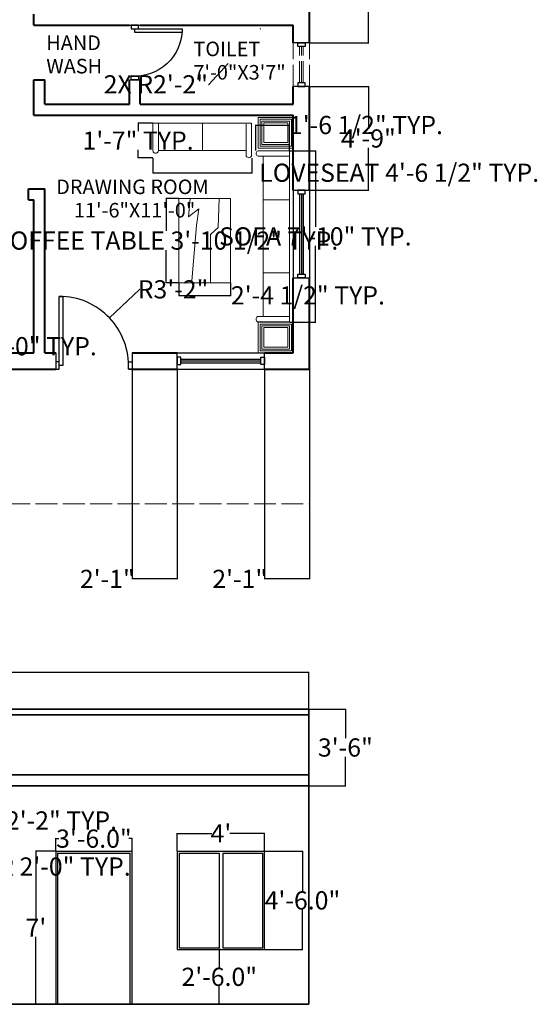
# Model space of a CAD drawing. Units: inches. Extents: x -413 to 212, y 1694 to 2633.
# Tile 3 of 5: x -98 to 187, y 1738 to 2279. Entities that reach past the tile are written whole.
import ezdxf

# ---------------------------------------------------------------- set-up
doc = ezdxf.new("R2010")
doc.units = ezdxf.units.IN
doc.header["$MEASUREMENT"] = 0
doc.linetypes.add('ACAD_ISO02W100', pattern=[15, 12, -3])
for name, color, linetype, lineweight in [('A-ANNO-DIMS', 5, 'Continuous', 18), ('A-AREA-IDEN', 251, 'Continuous', 25), ('A-ELEV', 20, 'Continuous', 35), ('A-ELEV-DOOR', 4, 'Continuous', 25), ('A-ELEV-GLAZ', 6, 'Continuous', 25), ('A-FLOR-OVHD', 20, 'ACAD_ISO02W100', 18), ('A-GLAZ-OVHD', 2, 'ACAD_ISO02W100', 18), ('A-GLAZ-VENT', 2, 'Continuous', 25), ('door', 4, 'Continuous', 25), ('furniture', 1, 'Continuous', 18), ('wall', 20, 'Continuous', 40), ('window', 6, 'Continuous', 25)]:
    doc.layers.add(name, color=color, linetype=linetype, lineweight=lineweight)
doc.styles.get("Standard").update_dxf_attribs({"font": 'arial.ttf'})
doc.dimstyles.get("Standard").update_dxf_attribs({"dimtxt": 10, "dimasz": 0.18, "dimexe": 0.18, "dimexo": 0.0625, "dimgap": 0.09, "dimtad": 0, "dimtih": 1, "dimtoh": 1, "dimdec": 1, "dimzin": 0, "dimdsep": 46, "dimlunit": 3, "dimtxsty": 'Standard', "dimblk": 'ARCHTICK', "dimcen": 0.09, "dimadec": 0, "dimazin": 0, "dimtfac": 1, "dimtdec": 1, "dimtofl": 0, "dimtmove": 0, "dimatfit": 3, "dimfxl": 1, "dimtolj": 1, "dimtzin": 0, "dimarcsym": 0})

# ---------------------------------------------------------------- blocks, each defined once
blk = doc.blocks.new('_ArchTick')
at = {"color": 0, "linetype": 'ByBlock', "const_width": 0.15}
blk.add_lwpolyline([(-0.5, -0.5), (0.5, 0.5)], dxfattribs=at)
blk = doc.blocks.new('*D4')
at = {"layer": 'A-ANNO-DIMS', "color": 0, "lineweight": -2, "transparency": 16777216}
for p, q in [((12.71, 1768.59), (11.69, 1768.59)), ((11.87, 1768.59), (11.87, 1758.78)), ((11.87, 1738.59), (11.87, 1748.39)), ((12.71, 1738.59), (11.69, 1738.59))]:
    blk.add_line(p, q, dxfattribs=at)
at = {"layer": 'Defpoints', "color": 0, "transparency": 16777216}
for p in [(12.77, 1768.59), (11.87, 1738.59), (12.77, 1738.59)]:
    blk.add_point(p, dxfattribs=at)
at = {"layer": 'A-ANNO-DIMS', "color": 0, "lineweight": -2, "transparency": 16777216, "xscale": 0.18, "yscale": 0.18, "zscale": 0.18}
for p, rotation in [((11.87, 1768.59), 90), ((11.87, 1738.59), 270)]:
    blk.add_blockref('_ArchTick', p, dxfattribs=dict(at, rotation=rotation))
at = {"layer": 'A-ANNO-DIMS', "color": 0, "transparency": 16777216, "insert": (11.87, 1753.59), "char_height": 10, "attachment_point": 5}
blk.add_mtext('\\A1;2\'-6.0"', dxfattribs=at)
blk = doc.blocks.new('*D5')
at = {"layer": 'A-ANNO-DIMS', "color": 0, "lineweight": -2, "transparency": 16777216}
for p, q in [((-78.04, 1822.59), (-89.03, 1822.59)), ((-88.85, 1822.59), (-88.85, 1785.68)), ((-88.85, 1738.59), (-88.85, 1775.5)), ((-78.04, 1738.59), (-89.03, 1738.59))]:
    blk.add_line(p, q, dxfattribs=at)
at = {"layer": 'Defpoints', "color": 0, "transparency": 16777216}
for p in [(-77.98, 1822.59), (-88.85, 1738.59), (-77.98, 1738.59)]:
    blk.add_point(p, dxfattribs=at)
at = {"layer": 'A-ANNO-DIMS', "color": 0, "lineweight": -2, "transparency": 16777216, "xscale": 0.18, "yscale": 0.18, "zscale": 0.18}
for p, rotation in [((-88.85, 1822.59), 90), ((-88.85, 1738.59), 270)]:
    blk.add_blockref('_ArchTick', p, dxfattribs=dict(at, rotation=rotation))
at = {"layer": 'A-ANNO-DIMS', "color": 0, "transparency": 16777216, "insert": (-88.85, 1780.59), "char_height": 10, "attachment_point": 5}
blk.add_mtext("\\A1;7'", dxfattribs=at)
blk = doc.blocks.new('*D6')
at = {"layer": 'A-ANNO-DIMS', "color": 0, "lineweight": -2, "transparency": 16777216}
for p, q in [((-77.98, 1822.65), (-77.98, 1829.7)), ((-77.98, 1829.52), (-76.18, 1829.52)), ((-35.98, 1829.52), (-37.77, 1829.52)), ((-35.98, 1822.65), (-35.98, 1829.7))]:
    blk.add_line(p, q, dxfattribs=at)
at = {"layer": 'Defpoints', "color": 0, "transparency": 16777216}
for p in [(-77.98, 1829.52), (-77.98, 1822.59), (-35.98, 1822.59)]:
    blk.add_point(p, dxfattribs=at)
at = {"layer": 'A-ANNO-DIMS', "color": 0, "lineweight": -2, "transparency": 16777216, "xscale": 0.18, "yscale": 0.18, "zscale": 0.18, "rotation": 180}
blk.add_blockref('_ArchTick', (-77.98, 1829.52), dxfattribs=at)
at = {"layer": 'A-ANNO-DIMS', "color": 0, "lineweight": -2, "transparency": 16777216, "xscale": 0.18, "yscale": 0.18, "zscale": 0.18}
blk.add_blockref('_ArchTick', (-35.98, 1829.52), dxfattribs=at)
at = {"layer": 'A-ANNO-DIMS', "color": 0, "transparency": 16777216, "insert": (-56.98, 1829.52), "char_height": 10, "attachment_point": 5}
blk.add_mtext('\\A1;3\'-6.0"', dxfattribs=at)
blk = doc.blocks.new('*D7')
at = {"layer": 'A-ANNO-DIMS', "color": 0, "lineweight": -2, "transparency": 16777216}
for p, q in [((36.84, 1822.59), (57.74, 1822.59)), ((57.56, 1822.59), (57.56, 1800.78)), ((57.56, 1768.59), (57.56, 1790.39)), ((36.84, 1768.59), (57.74, 1768.59))]:
    blk.add_line(p, q, dxfattribs=at)
at = {"layer": 'Defpoints', "color": 0, "transparency": 16777216}
for p in [(36.77, 1822.59), (36.77, 1768.59), (57.56, 1768.59)]:
    blk.add_point(p, dxfattribs=at)
at = {"layer": 'A-ANNO-DIMS', "color": 0, "lineweight": -2, "transparency": 16777216, "xscale": 0.18, "yscale": 0.18, "zscale": 0.18}
for p, rotation in [((57.56, 1822.59), 90), ((57.56, 1768.59), 270)]:
    blk.add_blockref('_ArchTick', p, dxfattribs=dict(at, rotation=rotation))
at = {"layer": 'A-ANNO-DIMS', "color": 0, "transparency": 16777216, "insert": (57.56, 1795.59), "char_height": 10, "attachment_point": 5}
blk.add_mtext('\\A1;4\'-6.0"', dxfattribs=at)
blk = doc.blocks.new('*D8')
at = {"layer": 'A-ANNO-DIMS', "color": 0, "lineweight": -2, "transparency": 16777216}
for p, q in [((-11.23, 1822.65), (-11.23, 1832.6)), ((-11.23, 1832.42), (7.88, 1832.42)), ((36.77, 1832.42), (17.67, 1832.42)), ((36.77, 1822.65), (36.77, 1832.6))]:
    blk.add_line(p, q, dxfattribs=at)
at = {"layer": 'Defpoints', "color": 0, "transparency": 16777216}
for p in [(-11.23, 1832.42), (-11.23, 1822.59), (36.77, 1822.59)]:
    blk.add_point(p, dxfattribs=at)
at = {"layer": 'A-ANNO-DIMS', "color": 0, "lineweight": -2, "transparency": 16777216, "xscale": 0.18, "yscale": 0.18, "zscale": 0.18, "rotation": 180}
blk.add_blockref('_ArchTick', (-11.23, 1832.42), dxfattribs=at)
at = {"layer": 'A-ANNO-DIMS', "color": 0, "lineweight": -2, "transparency": 16777216, "xscale": 0.18, "yscale": 0.18, "zscale": 0.18}
blk.add_blockref('_ArchTick', (36.77, 1832.42), dxfattribs=at)
at = {"layer": 'A-ANNO-DIMS', "color": 0, "transparency": 16777216, "insert": (12.77, 1832.42), "char_height": 10, "attachment_point": 5}
blk.add_mtext("\\A1;4'", dxfattribs=at)
blk = doc.blocks.new('WINDOW-48IN')
for p, q in [((0, 0), (0, 9)), ((0, 9), (48, 9)), ((2, 5.5), (46, 5.5)), ((48, 0), (48, 9)), ((2, 4.5), (46, 4.5)), ((2, 3.5), (46, 3.5)), ((0, 0), (48, 0))]:
    blk.add_line(p, q)
for points in [[(0, 2.5), (2, 2.5), (2, 6.5), (0, 6.5)], [(48, 2.5), (46, 2.5), (46, 6.5), (48, 6.5)]]:
    blk.add_lwpolyline(points, close=True)
blk = doc.blocks.new('VENT-JAMBS-24IN')
for p, q in [((0, 0), (0, 9)), ((24, 0), (24, 9))]:
    blk.add_line(p, q)
for points in [[(0, 2.5), (2, 2.5), (2, 6.5), (0, 6.5)], [(24, 2.5), (22, 2.5), (22, 6.5), (24, 6.5)]]:
    blk.add_lwpolyline(points, close=True)
blk = doc.blocks.new('VENT-PANEL-24IN')
for p, q in [((0, 9), (24, 9)), ((2, 5.5), (22, 5.5)), ((2, 4.5), (22, 4.5)), ((2, 3.5), (22, 3.5)), ((0, 0), (24, 0))]:
    blk.add_line(p, q)
blk = doc.blocks.new('DOOR-SWING-30IN')
for points in [[(0, 0), (0, 26), (-2, 26), (-2, 0)], [(-28, -2), (-26, -2), (-26, 2), (-28, 2)], [(2, -2), (0, -2), (0, 2), (2, 2)]]:
    blk.add_lwpolyline(points, close=True)
blk.add_arc((0, 0), 26, 90, 184.4117)
blk = doc.blocks.new('SOFA-THREE-SEAT')
for points in [[(0, 1.47), (0, 18.46), (94.05, 18.46), (94.05, 1.28)], [(3, 1.47), (3, 18.46)], [(27, 4), (27, 18.46)], [(67.05, 18.46), (67.05, 4)], [(91.05, 18.46), (91.05, 1.28)], [(91.05, 4), (3, 4)]]:
    blk.add_lwpolyline(points)
for centre, radius, start, end in [((1.5, 1.51), 1.5, 178.5982, 1.4018), ((92.55, 1.52), 1.52, 171.0874, 8.9126)]:
    blk.add_arc(centre, radius, start, end)
blk = doc.blocks.new('SOFA-TWO-SEAT')
for points in [[(0, 0), (0, 54.18), (17.18, 54.18)], [(0.47, 51.18), (17.65, 51.18)], [(14.93, 51.18), (14.93, 3.18)], [(0, 27.18), (14.93, 27.18)], [(15.01, 3), (0, 3)], [(0, 0), (14.93, 0)]]:
    blk.add_lwpolyline(points)
for centre, radius, start, end in [((17.41, 52.68), 1.52, 261.0874, 98.9126), ((14.97, 1.5), 1.5, 268.5982, 91.4018)]:
    blk.add_arc(centre, radius, start, end)
blk = doc.blocks.new('TABLE-COFFEE')
for p, q in [((0, 22.18), (0, 22.18)), ((0, 22.18), (15.93, 21.7)), ((15.93, 21.7), (19.8, 17.36)), ((19.8, 17.36), (46.35, 17.36)), ((10.14, 5.3), (5.79, 11.09)), ((5.79, 11.09), (14.97, 9.64)), ((0, 6.27), (0, 6.27)), ((0, 6.27), (10.14, 5.3)), ((14.97, 9.64), (45.38, 7.23))]:
    blk.add_line(p, q)
blk.add_lwpolyline([(0, 28.45), (46.35, 28.45), (46.35, 0), (0, 0)], close=True)
blk = doc.blocks.new('TABLE-END')
for points in [[(0, 19.24), (16.8, 19.24), (16.8, 0), (0, 0)], [(1, 18.24), (15.8, 18.24), (15.8, 1), (1, 1)], [(2, 17.24), (14.8, 17.24), (14.8, 2), (2, 2)], [(3, 16.24), (13.8, 16.24), (13.8, 3), (3, 3)]]:
    blk.add_lwpolyline(points, close=True)
blk = doc.blocks.new('*D31')
at = {"layer": 'A-ANNO-DIMS', "color": 0, "lineweight": -2, "transparency": 16777216}
for p, q in [((-179.98, 2096.55), (-179.98, 2100.26)), ((-179.98, 2100.08), (-155.98, 2100.08)), ((-155.98, 2096.55), (-155.98, 2100.26)), ((-155.98, 2100.08), (-155.8, 2100.08))]:
    blk.add_line(p, q, dxfattribs=at)
at = {"layer": 'Defpoints', "color": 0, "transparency": 16777216}
for p in [(-155.98, 2100.08), (-179.98, 2096.48), (-155.98, 2096.48)]:
    blk.add_point(p, dxfattribs=at)
at = {"layer": 'A-ANNO-DIMS', "color": 0, "lineweight": -2, "transparency": 16777216, "xscale": 0.18, "yscale": 0.18, "zscale": 0.18, "rotation": 180}
blk.add_blockref('_ArchTick', (-179.98, 2100.08), dxfattribs=at)
at = {"layer": 'A-ANNO-DIMS', "color": 0, "lineweight": -2, "transparency": 16777216, "xscale": 0.18, "yscale": 0.18, "zscale": 0.18}
blk.add_blockref('_ArchTick', (-155.98, 2100.08), dxfattribs=at)
at = {"layer": 'A-ANNO-DIMS', "color": 0, "transparency": 16777216, "insert": (-104.4, 2100.08), "char_height": 10, "attachment_point": 5}
blk.add_mtext('\\A1;VENT 2\'-0" TYP.', dxfattribs=at)
blk = doc.blocks.new('*D45')
at = {"layer": 'A-ANNO-DIMS', "color": 0, "lineweight": -2, "transparency": 16777216}
for p, q in [((50.59, 2207.49), (64.83, 2207.49)), ((64.65, 2207.49), (64.65, 2165.68)), ((64.65, 2113.33), (64.65, 2155.15)), ((50.59, 2113.33), (64.83, 2113.33))]:
    blk.add_line(p, q, dxfattribs=at)
at = {"layer": 'Defpoints', "color": 0, "transparency": 16777216}
for p in [(50.52, 2207.49), (50.52, 2113.33), (64.65, 2113.33)]:
    blk.add_point(p, dxfattribs=at)
at = {"layer": 'A-ANNO-DIMS', "color": 0, "lineweight": -2, "transparency": 16777216, "xscale": 0.18, "yscale": 0.18, "zscale": 0.18}
for p, rotation in [((64.65, 2207.49), 90), ((64.65, 2113.33), 270)]:
    blk.add_blockref('_ArchTick', p, dxfattribs=dict(at, rotation=rotation))
at = {"layer": 'A-ANNO-DIMS', "color": 0, "transparency": 16777216, "insert": (64.65, 2160.41), "char_height": 10, "attachment_point": 5}
blk.add_mtext('\\A1;SOFA 7\'-10" TYP.', dxfattribs=at)
blk = doc.blocks.new('*D46')
at = {"layer": 'A-ANNO-DIMS', "color": 0, "lineweight": -2, "transparency": 16777216}
for p, q in [((31.98, 2207.55), (31.98, 2221.79)), ((31.98, 2221.61), (50.52, 2221.61)), ((50.52, 2207.55), (50.52, 2221.79)), ((50.52, 2221.61), (50.7, 2221.61))]:
    blk.add_line(p, q, dxfattribs=at)
at = {"layer": 'Defpoints', "color": 0, "transparency": 16777216}
for p in [(50.52, 2221.61), (31.98, 2207.49), (50.52, 2207.49)]:
    blk.add_point(p, dxfattribs=at)
at = {"layer": 'A-ANNO-DIMS', "color": 0, "lineweight": -2, "transparency": 16777216, "xscale": 0.18, "yscale": 0.18, "zscale": 0.18, "rotation": 180}
blk.add_blockref('_ArchTick', (31.98, 2221.61), dxfattribs=at)
at = {"layer": 'A-ANNO-DIMS', "color": 0, "lineweight": -2, "transparency": 16777216, "xscale": 0.18, "yscale": 0.18, "zscale": 0.18}
blk.add_blockref('_ArchTick', (50.52, 2221.61), dxfattribs=at)
at = {"layer": 'A-ANNO-DIMS', "color": 0, "transparency": 16777216, "insert": (92.45, 2221.61), "char_height": 10, "attachment_point": 5}
blk.add_mtext('\\A1;1\'-6 1/2" TYP.', dxfattribs=at)
blk = doc.blocks.new('*D47')
at = {"layer": 'A-ANNO-DIMS', "color": 0, "lineweight": -2, "transparency": 16777216}
for p, q in [((-24.57, 2203.48), (-24.57, 2195.22)), ((29.72, 2203.48), (29.72, 2195.22)), ((-24.57, 2195.4), (29.72, 2195.4)), ((29.72, 2195.4), (29.9, 2195.4))]:
    blk.add_line(p, q, dxfattribs=at)
at = {"layer": 'Defpoints', "color": 0, "transparency": 16777216}
for p in [(-24.57, 2203.54), (29.72, 2203.54), (29.72, 2195.4)]:
    blk.add_point(p, dxfattribs=at)
at = {"layer": 'A-ANNO-DIMS', "color": 0, "lineweight": -2, "transparency": 16777216, "xscale": 0.18, "yscale": 0.18, "zscale": 0.18, "rotation": 180}
blk.add_blockref('_ArchTick', (-24.57, 2195.4), dxfattribs=at)
at = {"layer": 'A-ANNO-DIMS', "color": 0, "lineweight": -2, "transparency": 16777216, "xscale": 0.18, "yscale": 0.18, "zscale": 0.18}
blk.add_blockref('_ArchTick', (29.72, 2195.4), dxfattribs=at)
at = {"layer": 'A-ANNO-DIMS', "color": 0, "transparency": 16777216, "insert": (110.71, 2195.4), "char_height": 10, "attachment_point": 5}
blk.add_mtext('\\A1;LOVESEAT 4\'-6 1/2" TYP.', dxfattribs=at)
blk = doc.blocks.new('*D48')
at = {"layer": 'A-ANNO-DIMS', "color": 0, "lineweight": -2, "transparency": 16777216}
for p, q in [((-24.63, 2222.56), (-32.89, 2222.56)), ((-32.71, 2222.56), (-32.71, 2218.16)), ((-32.71, 2203.54), (-32.71, 2207.94)), ((-24.63, 2203.54), (-32.89, 2203.54))]:
    blk.add_line(p, q, dxfattribs=at)
at = {"layer": 'Defpoints', "color": 0, "transparency": 16777216}
for p in [(-24.57, 2222.56), (-32.71, 2203.54), (-24.57, 2203.54)]:
    blk.add_point(p, dxfattribs=at)
at = {"layer": 'A-ANNO-DIMS', "color": 0, "lineweight": -2, "transparency": 16777216, "xscale": 0.18, "yscale": 0.18, "zscale": 0.18}
for p, rotation in [((-32.71, 2222.56), 90), ((-32.71, 2203.54), 270)]:
    blk.add_blockref('_ArchTick', p, dxfattribs=dict(at, rotation=rotation))
at = {"layer": 'A-ANNO-DIMS', "color": 0, "transparency": 16777216, "insert": (-32.71, 2213.05), "char_height": 10, "attachment_point": 5}
blk.add_mtext('\\A1;1\'-7" TYP.', dxfattribs=at)
blk = doc.blocks.new('*D49')
at = {"layer": 'A-ANNO-DIMS', "color": 0, "lineweight": -2, "transparency": 16777216}
for p, q in [((-10.42, 2181.31), (-17.49, 2181.31)), ((-17.31, 2181.31), (-17.31, 2163.4)), ((-17.31, 2134.96), (-17.31, 2152.87)), ((-10.42, 2134.96), (-17.49, 2134.96))]:
    blk.add_line(p, q, dxfattribs=at)
at = {"layer": 'Defpoints', "color": 0, "transparency": 16777216}
for p in [(-10.36, 2181.31), (-17.31, 2134.96), (-10.36, 2134.96)]:
    blk.add_point(p, dxfattribs=at)
at = {"layer": 'A-ANNO-DIMS', "color": 0, "lineweight": -2, "transparency": 16777216, "xscale": 0.18, "yscale": 0.18, "zscale": 0.18}
for p, rotation in [((-17.31, 2181.31), 90), ((-17.31, 2134.96), 270)]:
    blk.add_blockref('_ArchTick', p, dxfattribs=dict(at, rotation=rotation))
at = {"layer": 'A-ANNO-DIMS', "color": 0, "transparency": 16777216, "insert": (-17.31, 2158.13), "char_height": 10, "attachment_point": 5}
blk.add_mtext('\\A1;COFFEE TABLE 3\'-10 1/2" TYP.', dxfattribs=at)
blk = doc.blocks.new('*D50')
at = {"layer": 'A-ANNO-DIMS', "color": 0, "lineweight": -2, "transparency": 16777216}
for p, q in [((-10.36, 2134.9), (-10.36, 2127.83)), ((18.09, 2134.9), (18.09, 2127.83)), ((-10.36, 2128.01), (18.09, 2128.01)), ((18.09, 2128.01), (18.27, 2128.01))]:
    blk.add_line(p, q, dxfattribs=at)
at = {"layer": 'Defpoints', "color": 0, "transparency": 16777216}
for p in [(-10.36, 2134.96), (18.09, 2134.96), (18.09, 2128.01)]:
    blk.add_point(p, dxfattribs=at)
at = {"layer": 'A-ANNO-DIMS', "color": 0, "lineweight": -2, "transparency": 16777216, "xscale": 0.18, "yscale": 0.18, "zscale": 0.18, "rotation": 180}
blk.add_blockref('_ArchTick', (-10.36, 2128.01), dxfattribs=at)
at = {"layer": 'A-ANNO-DIMS', "color": 0, "lineweight": -2, "transparency": 16777216, "xscale": 0.18, "yscale": 0.18, "zscale": 0.18}
blk.add_blockref('_ArchTick', (18.09, 2128.01), dxfattribs=at)
at = {"layer": 'A-ANNO-DIMS', "color": 0, "transparency": 16777216, "insert": (60.57, 2128.01), "char_height": 10, "attachment_point": 5}
blk.add_mtext('\\A1;2\'-4 1/2" TYP.', dxfattribs=at)
blk = doc.blocks.new('*D53')
at = {"layer": 'A-ANNO-DIMS', "color": 0, "lineweight": -2, "transparency": 16777216}
for p, q in [((-180.98, 1835.65), (-180.98, 1839.67)), ((-180.98, 1839.49), (-154.98, 1839.49)), ((-154.98, 1835.65), (-154.98, 1839.67)), ((-154.98, 1839.49), (-154.8, 1839.49))]:
    blk.add_line(p, q, dxfattribs=at)
at = {"layer": 'Defpoints', "color": 0, "transparency": 16777216}
for p in [(-154.98, 1839.49), (-180.98, 1835.59), (-154.98, 1835.59)]:
    blk.add_point(p, dxfattribs=at)
at = {"layer": 'A-ANNO-DIMS', "color": 0, "lineweight": -2, "transparency": 16777216, "xscale": 0.18, "yscale": 0.18, "zscale": 0.18, "rotation": 180}
blk.add_blockref('_ArchTick', (-180.98, 1839.49), dxfattribs=at)
at = {"layer": 'A-ANNO-DIMS', "color": 0, "lineweight": -2, "transparency": 16777216, "xscale": 0.18, "yscale": 0.18, "zscale": 0.18}
blk.add_blockref('_ArchTick', (-154.98, 1839.49), dxfattribs=at)
at = {"layer": 'A-ANNO-DIMS', "color": 0, "transparency": 16777216, "insert": (-98.12, 1839.49), "char_height": 10, "attachment_point": 5}
blk.add_mtext('\\A1;FRAME 2\'-2" TYP.', dxfattribs=at)
blk = doc.blocks.new('*D55')
at = {"layer": 'A-ANNO-DIMS', "color": 0, "lineweight": -2, "transparency": 16777216}
for p, q in [((-179.98, 1817.73), (-179.98, 1814.01)), ((-179.98, 1814.19), (-155.98, 1814.19)), ((-155.98, 1817.73), (-155.98, 1814.01)), ((-155.98, 1814.19), (-155.8, 1814.19))]:
    blk.add_line(p, q, dxfattribs=at)
at = {"layer": 'Defpoints', "color": 0, "transparency": 16777216}
for p in [(-179.98, 1817.79), (-155.98, 1817.79), (-155.98, 1814.19)]:
    blk.add_point(p, dxfattribs=at)
at = {"layer": 'A-ANNO-DIMS', "color": 0, "lineweight": -2, "transparency": 16777216, "xscale": 0.18, "yscale": 0.18, "zscale": 0.18, "rotation": 180}
blk.add_blockref('_ArchTick', (-179.98, 1814.19), dxfattribs=at)
at = {"layer": 'A-ANNO-DIMS', "color": 0, "lineweight": -2, "transparency": 16777216, "xscale": 0.18, "yscale": 0.18, "zscale": 0.18}
blk.add_blockref('_ArchTick', (-155.98, 1814.19), dxfattribs=at)
at = {"layer": 'A-ANNO-DIMS', "color": 0, "transparency": 16777216, "insert": (-94.78, 1814.19), "char_height": 10, "attachment_point": 5}
blk.add_mtext('\\A1;LOUVER 2\'-0" TYP.', dxfattribs=at)
blk = doc.blocks.new('*D60')
at = {"layer": 'A-ANNO-DIMS', "color": 0, "lineweight": -2, "transparency": 16777216}
for p, q in [((-338.98, 1900.65), (-338.98, 1920.92)), ((-338.98, 1920.74), (-156.26, 1920.74)), ((60.99, 1920.74), (-121.73, 1920.74)), ((60.99, 1900.65), (60.99, 1920.92))]:
    blk.add_line(p, q, dxfattribs=at)
at = {"layer": 'Defpoints', "color": 0, "transparency": 16777216}
for p in [(60.99, 1920.74), (-338.98, 1900.59), (60.99, 1900.59)]:
    blk.add_point(p, dxfattribs=at)
at = {"layer": 'A-ANNO-DIMS', "color": 0, "lineweight": -2, "transparency": 16777216, "xscale": 0.18, "yscale": 0.18, "zscale": 0.18, "rotation": 180}
blk.add_blockref('_ArchTick', (-338.98, 1920.74), dxfattribs=at)
at = {"layer": 'A-ANNO-DIMS', "color": 0, "lineweight": -2, "transparency": 16777216, "xscale": 0.18, "yscale": 0.18, "zscale": 0.18}
blk.add_blockref('_ArchTick', (60.99, 1920.74), dxfattribs=at)
at = {"layer": 'A-ANNO-DIMS', "color": 0, "transparency": 16777216, "insert": (-139, 1920.74), "char_height": 10, "attachment_point": 5}
blk.add_mtext('\\A1;33\'-4"', dxfattribs=at)
blk = doc.blocks.new('*D62')
at = {"layer": 'A-ANNO-DIMS', "color": 0, "lineweight": -2, "transparency": 16777216}
for p, q in [((61.05, 1900.59), (81.32, 1900.59)), ((81.14, 1900.59), (81.14, 1884.79)), ((81.14, 1858.59), (81.14, 1874.39)), ((61.05, 1858.59), (81.32, 1858.59))]:
    blk.add_line(p, q, dxfattribs=at)
at = {"layer": 'Defpoints', "color": 0, "transparency": 16777216}
for p in [(60.99, 1900.59), (81.14, 1900.59), (60.99, 1858.59)]:
    blk.add_point(p, dxfattribs=at)
at = {"layer": 'A-ANNO-DIMS', "color": 0, "lineweight": -2, "transparency": 16777216, "xscale": 0.18, "yscale": 0.18, "zscale": 0.18}
for p, rotation in [((81.14, 1900.59), 90), ((81.14, 1858.59), 270)]:
    blk.add_blockref('_ArchTick', p, dxfattribs=dict(at, rotation=rotation))
at = {"layer": 'A-ANNO-DIMS', "color": 0, "transparency": 16777216, "insert": (81.14, 1879.59), "char_height": 10, "attachment_point": 5}
blk.add_mtext('\\A1;3\'-6"', dxfattribs=at)
blk = doc.blocks.new('*D72')
at = {"layer": 'A-ANNO-DIMS', "color": 0, "lineweight": -2, "transparency": 16777216}
for p, q in [((61.59, 2312.48), (93.95, 2312.48)), ((93.77, 2312.48), (93.77, 2294.81)), ((93.77, 2266.73), (93.77, 2284.41)), ((61.59, 2266.73), (93.95, 2266.73))]:
    blk.add_line(p, q, dxfattribs=at)
at = {"layer": 'Defpoints', "color": 0, "transparency": 16777216}
for p in [(61.52, 2312.48), (61.52, 2266.73), (93.77, 2266.73)]:
    blk.add_point(p, dxfattribs=at)
at = {"layer": 'A-ANNO-DIMS', "color": 0, "lineweight": -2, "transparency": 16777216, "xscale": 0.18, "yscale": 0.18, "zscale": 0.18}
for p, rotation in [((93.77, 2312.48), 90), ((93.77, 2266.73), 270)]:
    blk.add_blockref('_ArchTick', p, dxfattribs=dict(at, rotation=rotation))
at = {"layer": 'A-ANNO-DIMS', "color": 0, "transparency": 16777216, "insert": (93.77, 2289.61), "char_height": 10, "attachment_point": 5}
blk.add_mtext('\\A1;3\'-10"', dxfattribs=at)
blk = doc.blocks.new('*D73')
at = {"layer": 'A-ANNO-DIMS', "color": 0, "lineweight": -2, "transparency": 16777216}
for p, q in [((61.59, 2242.73), (93.95, 2242.73)), ((93.77, 2242.73), (93.77, 2219.43)), ((93.77, 2185.73), (93.77, 2209.04)), ((61.59, 2185.73), (93.95, 2185.73))]:
    blk.add_line(p, q, dxfattribs=at)
at = {"layer": 'Defpoints', "color": 0, "transparency": 16777216}
for p in [(61.52, 2242.73), (61.52, 2185.73), (93.77, 2185.73)]:
    blk.add_point(p, dxfattribs=at)
at = {"layer": 'A-ANNO-DIMS', "color": 0, "lineweight": -2, "transparency": 16777216, "xscale": 0.18, "yscale": 0.18, "zscale": 0.18}
for p, rotation in [((93.77, 2242.73), 90), ((93.77, 2185.73), 270)]:
    blk.add_blockref('_ArchTick', p, dxfattribs=dict(at, rotation=rotation))
at = {"layer": 'A-ANNO-DIMS', "color": 0, "transparency": 16777216, "insert": (93.77, 2214.23), "char_height": 10, "attachment_point": 5}
blk.add_mtext('\\A1;4\'-9"', dxfattribs=at)
blk = doc.blocks.new('*D74')
at = {"layer": 'A-ANNO-DIMS', "color": 0, "lineweight": -2, "transparency": 16777216}
for p, q in [((36.77, 2087.42), (36.77, 1972.05)), ((61.52, 2087.42), (61.52, 1972.05)), ((36.77, 1972.23), (36.59, 1972.23)), ((61.52, 1972.23), (36.77, 1972.23))]:
    blk.add_line(p, q, dxfattribs=at)
at = {"layer": 'Defpoints', "color": 0, "transparency": 16777216}
for p in [(36.77, 2087.48), (61.52, 2087.48), (36.77, 1972.23)]:
    blk.add_point(p, dxfattribs=at)
at = {"layer": 'A-ANNO-DIMS', "color": 0, "lineweight": -2, "transparency": 16777216, "xscale": 0.18, "yscale": 0.18, "zscale": 0.18, "rotation": 180}
blk.add_blockref('_ArchTick', (36.77, 1972.23), dxfattribs=at)
at = {"layer": 'A-ANNO-DIMS', "color": 0, "lineweight": -2, "transparency": 16777216, "xscale": 0.18, "yscale": 0.18, "zscale": 0.18}
blk.add_blockref('_ArchTick', (61.52, 1972.23), dxfattribs=at)
at = {"layer": 'A-ANNO-DIMS', "color": 0, "transparency": 16777216, "insert": (23.13, 1972.23), "char_height": 10, "attachment_point": 5}
blk.add_mtext('\\A1;2\'-1"', dxfattribs=at)
blk = doc.blocks.new('*D75')
at = {"layer": 'A-ANNO-DIMS', "color": 0, "lineweight": -2, "transparency": 16777216}
for p, q in [((-35.98, 2087.42), (-35.98, 1972.05)), ((-11.23, 2087.42), (-11.23, 1972.05)), ((-35.98, 1972.23), (-36.16, 1972.23)), ((-11.23, 1972.23), (-35.98, 1972.23))]:
    blk.add_line(p, q, dxfattribs=at)
at = {"layer": 'Defpoints', "color": 0, "transparency": 16777216}
for p in [(-35.98, 2087.48), (-11.23, 2087.48), (-35.98, 1972.23)]:
    blk.add_point(p, dxfattribs=at)
at = {"layer": 'A-ANNO-DIMS', "color": 0, "lineweight": -2, "transparency": 16777216, "xscale": 0.18, "yscale": 0.18, "zscale": 0.18, "rotation": 180}
blk.add_blockref('_ArchTick', (-35.98, 1972.23), dxfattribs=at)
at = {"layer": 'A-ANNO-DIMS', "color": 0, "lineweight": -2, "transparency": 16777216, "xscale": 0.18, "yscale": 0.18, "zscale": 0.18}
blk.add_blockref('_ArchTick', (-11.23, 1972.23), dxfattribs=at)
at = {"layer": 'A-ANNO-DIMS', "color": 0, "transparency": 16777216, "insert": (-49.62, 1972.23), "char_height": 10, "attachment_point": 5}
blk.add_mtext('\\A1;2\'-1"', dxfattribs=at)
blk = doc.blocks.new('*D82')
at = {"layer": 'A-ANNO-DIMS', "color": 0, "lineweight": -2, "transparency": 16777216}
for p, q in [((-31.87, 2131.33), (-48.41, 2115.64)), ((-31.69, 2131.33), (-31.87, 2131.33)), ((-76.07, 2089.48), (-75.89, 2089.48)), ((-75.98, 2089.39), (-75.98, 2089.57))]:
    blk.add_line(p, q, dxfattribs=at)
at = {"layer": 'Defpoints', "color": 0, "transparency": 16777216}
for p in [(-48.41, 2115.64), (-75.98, 2089.48)]:
    blk.add_point(p, dxfattribs=at)
at = {"layer": 'A-ANNO-DIMS', "color": 0, "lineweight": -2, "transparency": 16777216, "xscale": 0.18, "yscale": 0.18, "zscale": 0.18, "rotation": 223.4920055402341}
blk.add_blockref('_ArchTick', (-48.41, 2115.64), dxfattribs=at)
at = {"layer": 'A-ANNO-DIMS', "color": 0, "transparency": 16777216, "insert": (-13.52, 2131.33), "char_height": 10, "attachment_point": 5}
blk.add_mtext('\\A1;R3\'-2"', dxfattribs=at)
blk = doc.blocks.new('*D84')
at = {"layer": 'A-ANNO-DIMS', "color": 0, "lineweight": -2, "transparency": 16777216}
for p, q in [((34.39, 2274.48), (34.57, 2274.48)), ((34.48, 2274.39), (34.48, 2274.57)), ((6.21, 2243.96), (16.81, 2255.41)), ((6.03, 2243.96), (6.21, 2243.96))]:
    blk.add_line(p, q, dxfattribs=at)
at = {"layer": 'Defpoints', "color": 0, "transparency": 16777216}
for p in [(34.48, 2274.48), (16.81, 2255.41)]:
    blk.add_point(p, dxfattribs=at)
at = {"layer": 'A-ANNO-DIMS', "color": 0, "lineweight": -2, "transparency": 16777216, "xscale": 0.18, "yscale": 0.18, "zscale": 0.18, "rotation": 47.20531037035683}
blk.add_blockref('_ArchTick', (16.81, 2255.41), dxfattribs=at)
at = {"layer": 'A-ANNO-DIMS', "color": 0, "transparency": 16777216, "insert": (-22.96, 2243.96), "char_height": 10, "attachment_point": 5}
blk.add_mtext('\\A1;2X R2\'-2"', dxfattribs=at)

msp = doc.modelspace()

# ---------------------------------------------------------------- linework, layer by layer
at = {"layer": 'A-ELEV'}
for p, q in [((-338.98, 1900.59), (60.99, 1900.59)), ((60.99, 1900.59), (60.99, 1738.59)), ((-293.98, 1897.59), (60.99, 1897.59)), ((-293.98, 1864.59), (60.99, 1864.59)), ((-192.52, 1858.59), (60.99, 1858.59)), ((-338.98, 1738.59), (60.99, 1738.59))]:
    msp.add_line(p, q, dxfattribs=at)
at = {"layer": 'A-ELEV-DOOR'}
for p, q in [((-77.98, 1822.59), (-35.98, 1822.59)), ((-77.98, 1822.59), (-77.98, 1738.59)), ((-76.98, 1821.59), (-36.98, 1821.59)), ((-76.98, 1821.59), (-76.98, 1738.59)), ((-36.98, 1738.59), (-36.98, 1821.59)), ((-35.98, 1738.59), (-35.98, 1822.59)), ((-77.98, 1738.59), (-76.98, 1738.59)), ((-36.98, 1738.59), (-35.98, 1738.59))]:
    msp.add_line(p, q, dxfattribs=at)
at = {"layer": 'A-ELEV-GLAZ'}
for p, q in [((-11.23, 1822.59), (36.77, 1822.59)), ((-11.23, 1822.59), (-11.23, 1768.59)), ((-10.23, 1821.59), (11.77, 1821.59)), ((-10.23, 1821.59), (-10.23, 1769.59)), ((11.77, 1821.59), (11.77, 1769.59)), ((13.77, 1821.59), (13.77, 1769.59)), ((13.77, 1821.59), (35.77, 1821.59)), ((35.77, 1769.59), (35.77, 1821.59)), ((36.77, 1768.59), (36.77, 1822.59)), ((-10.23, 1769.59), (11.77, 1769.59)), ((13.77, 1769.59), (35.77, 1769.59)), ((-11.23, 1768.59), (36.77, 1768.59))]:
    msp.add_line(p, q, dxfattribs=at)
at = {"layer": 'A-FLOR-OVHD'}
for p, q in [((61.52, 2013.48), (61.52, 2087.48)), ((-193.98, 2013.48), (61.52, 2013.48))]:
    msp.add_line(p, q, dxfattribs=at)
at = {"layer": 'door'}
for p, q in [((-37.48, 2276.48), (-31.48, 2276.48)), ((-37.48, 2246.48), (-31.48, 2246.48)), ((-77.98, 2096.48), (-77.98, 2087.48)), ((-35.98, 2096.48), (-35.98, 2087.48)), ((-77.98, 2087.48), (-75.98, 2087.48)), ((-38.03, 2087.48), (-35.98, 2087.48))]:
    msp.add_line(p, q, dxfattribs=at)
for points in [[(-75.98, 2089.48), (-75.98, 2127.48), (-73.98, 2127.48), (-73.98, 2089.48)], [(-77.98, 2087.48), (-75.98, 2087.48), (-75.98, 2091.48), (-77.98, 2091.48)], [(-35.98, 2087.48), (-37.98, 2087.48), (-37.98, 2091.48), (-35.98, 2091.48)]]:
    msp.add_lwpolyline(points, close=True, dxfattribs=at)
msp.add_arc((-75.98, 2089.48), 38, 356.983, 90, dxfattribs=at)
at = {"layer": 'wall'}
for p, q in [((61.52, 2266.73), (61.52, 2312.48)), ((-89.98, 2276.48), (-89.98, 2282.48)), ((-89.98, 2276.48), (-37.48, 2276.48)), ((-31.48, 2276.48), (52.52, 2276.48)), ((52.52, 2266.73), (52.52, 2276.48)), ((-89.98, 2226.98), (-89.98, 2246.48)), ((-89.98, 2246.48), (-83.98, 2246.48)), ((-83.98, 2232.98), (-83.98, 2246.48)), ((-37.48, 2232.98), (-37.48, 2246.48)), ((-31.48, 2232.98), (-31.48, 2246.48)), ((52.52, 2232.98), (52.52, 2242.73)), ((61.52, 2185.73), (61.52, 2242.73)), ((-83.98, 2232.98), (-37.48, 2232.98)), ((-31.48, 2232.98), (52.52, 2232.98)), ((-89.98, 2226.98), (52.52, 2226.98)), ((52.52, 2185.73), (52.52, 2226.98)), ((-92.98, 2180.48), (-92.98, 2186.48)), ((-92.98, 2186.48), (-83.98, 2186.48)), ((-83.98, 2096.48), (-83.98, 2186.48)), ((-92.98, 2180.48), (-89.98, 2180.48)), ((-89.98, 2096.48), (-89.98, 2180.48)), ((52.52, 2096.48), (52.52, 2137.73)), ((61.52, 2087.48), (61.52, 2137.73)), ((-101.98, 2096.48), (-89.98, 2096.48)), ((-83.98, 2096.48), (-77.98, 2096.48)), ((-35.98, 2096.48), (-11.23, 2096.48)), ((36.77, 2096.48), (52.52, 2096.48)), ((-101.98, 2087.48), (-77.98, 2087.48)), ((-35.98, 2087.48), (-11.23, 2087.48)), ((36.77, 2087.48), (61.52, 2087.48))]:
    msp.add_line(p, q, dxfattribs=at)

# ---------------------------------------------------------------- block references
at = {"layer": 'A-GLAZ-OVHD', "rotation": 90.0000000000019}
msp.add_blockref('VENT-PANEL-24IN', (61.52, 2242.73), dxfattribs=at)
at = {"layer": 'A-GLAZ-VENT', "rotation": 89.99999999999852}
msp.add_blockref('VENT-JAMBS-24IN', (61.52, 2242.73), dxfattribs=at)
at = {"layer": 'door', "extrusion": (0, 0, -1), "zscale": -1, "rotation": 89.99999999999795}
msp.add_blockref('DOOR-SWING-30IN', (34.48, 2274.48), dxfattribs=at)
at = {"layer": 'furniture'}
for name, p, rotation in [('TABLE-END', (33.28, 2225.78), 269.999999999998), ('SOFA-TWO-SEAT', (-24.56, 2222.56), 270.0000000000001), ('SOFA-THREE-SEAT', (32.06, 2207.48), 269.999999999999), ('TABLE-COFFEE', (-10.36, 2181.31), 270.0000000000003), ('TABLE-END', (33.28, 2113.28), 269.999999999998)]:
    msp.add_blockref(name, p, dxfattribs=dict(at, rotation=rotation))
at = {"layer": 'window', "rotation": 270.0000000000045}
msp.add_blockref('WINDOW-48IN', (52.52, 2185.73), dxfattribs=at)
at = {"layer": 'window'}
msp.add_blockref('WINDOW-48IN', (-11.23, 2087.49), dxfattribs=at)

# ---------------------------------------------------------------- texts
at = {"layer": 'A-AREA-IDEN'}
for s, p in [('HAND ', (-83.13, 2262.8)), ('TOILET', (-2.32, 2259.42)), ('WASH', (-83.13, 2249.95)), ('7\'-0"X3\'7"', (-2.32, 2246.57)), ('DRAWING ROOM', (-77.69, 2183.66)), ('    11\'-6"X11\'-0"', (-77.69, 2170.81))]:
    msp.add_text(s, height=8, dxfattribs=at).set_placement(p)

# ---------------------------------------------------------------- dimensions: what is measured, and where the dimension line sits
at = {"layer": 'A-ANNO-DIMS'}
for base, p1, p2, override, picture, middle in [((93.774334, 2266.734571), (61.524334, 2312.484571), (61.524334, 2266.734571), {"dimdec": 1, "dimlfac": 1, "dimrnd": 0, "dimzin": 1, "dimdsep": 46, "dimlunit": 4, "dimfrac": 2}, '*D72', (93.774334, 2289.609571)), ((93.77, 2185.73), (61.52, 2242.73), (61.52, 2185.73), {"dimdec": 1, "dimlfac": 1, "dimrnd": 0, "dimzin": 1, "dimdsep": 46, "dimlunit": 4, "dimfrac": 2}, '*D73', (93.77, 2214.23)), ((81.14, 1900.59), (60.99, 1858.59), (60.99, 1900.59), {"dimdec": 1, "dimlfac": 1, "dimrnd": 0, "dimzin": 1, "dimdsep": 46, "dimlunit": 4, "dimfrac": 2}, '*D62', (81.14, 1879.59)), ((-88.85, 1738.59), (-77.98, 1822.59), (-77.98, 1738.59), {"dimclrd": 0, "dimclre": 0, "dimclrt": 0}, '*D5', (-88.85, 1780.59)), ((57.56, 1768.59), (36.77, 1822.59), (36.77, 1768.59), {"dimclrd": 0, "dimclre": 0, "dimclrt": 0}, '*D7', (57.56, 1795.59)), ((11.87, 1738.59), (12.77, 1768.59), (12.77, 1738.59), {"dimclrd": 0, "dimclre": 0, "dimclrt": 0}, '*D4', (11.87, 1753.59))]:
    dim = msp.add_linear_dim(base=base, p1=p1, p2=p2, angle=90, dimstyle='Standard', override=override, dxfattribs=at)
    dim.commit()
    dim.dimension.update_dxf_attribs({"geometry": picture, "text_midpoint": middle})
dim = msp.add_radius_dim(center=(34.48, 2274.48), mpoint=(16.81, 2255.41), text='2X <>', dimstyle='Standard', override={"dimdec": 1, "dimlfac": 1, "dimrnd": 0, "dimzin": 1, "dimdsep": 46, "dimlunit": 4, "dimfrac": 2}, dxfattribs=at)
dim.commit()
dim.dimension.update_dxf_attribs({"geometry": '*D84', "text_midpoint": (-22.96, 2243.96), "dimtype": 164})
for base, p1, p2, text, picture, middle in [((50.52, 2221.61), (31.98, 2207.49), (50.52, 2207.49), '<> TYP.', '*D46', (92.45, 2221.61)), ((29.72, 2195.4), (-24.57, 2203.54), (29.72, 2203.54), 'LOVESEAT <> TYP.', '*D47', (110.71, 2195.4)), ((18.0909, 2128.0075), (-10.3595, 2134.9599), (18.0909, 2134.9599), '<> TYP.', '*D50', (60.5745, 2128.0075)), ((-155.98, 2100.08), (-179.98, 2096.48), (-155.98, 2096.48), 'VENT <> TYP.', '*D31', (-104.4, 2100.08)), ((-154.98, 1839.49), (-180.98, 1835.59), (-154.98, 1835.59), 'FRAME <> TYP.', '*D53', (-98.12, 1839.49)), ((-155.98, 1814.19), (-179.98, 1817.79), (-155.98, 1817.79), 'LOUVER <> TYP.', '*D55', (-94.78, 1814.19))]:
    dim = msp.add_linear_dim(base=base, p1=p1, p2=p2, text=text, dimstyle='Standard', override={"dimdec": 1, "dimlfac": 1, "dimrnd": 0, "dimzin": 1, "dimdsep": 46, "dimlunit": 4, "dimfrac": 2}, dxfattribs=at)
    dim.commit()
    dim.dimension.update_dxf_attribs({"geometry": picture, "text_midpoint": middle})
for base, p1, p2, text, picture, middle in [((-32.71, 2203.54), (-24.57, 2222.56), (-24.57, 2203.54), '<> TYP.', '*D48', (-32.71, 2213.05)), ((64.65, 2113.33), (50.52, 2207.49), (50.52, 2113.33), 'SOFA <> TYP.', '*D45', (64.65, 2160.41)), ((-17.312, 2134.9599), (-10.3595, 2181.3098), (-10.3595, 2134.9599), 'COFFEE TABLE <> TYP.', '*D49', (-17.312, 2158.1349))]:
    dim = msp.add_linear_dim(base=base, p1=p1, p2=p2, angle=270, text=text, dimstyle='Standard', override={"dimdec": 1, "dimlfac": 1, "dimrnd": 0, "dimzin": 1, "dimdsep": 46, "dimlunit": 4, "dimfrac": 2}, dxfattribs=at)
    dim.commit()
    dim.dimension.update_dxf_attribs({"geometry": picture, "text_midpoint": middle})
dim = msp.add_radius_dim(center=(-75.98, 2089.48), mpoint=(-48.41, 2115.64), dimstyle='Standard', override={"dimdec": 1, "dimlfac": 1, "dimrnd": 0, "dimzin": 1, "dimdsep": 46, "dimlunit": 4, "dimfrac": 2}, dxfattribs=at)
dim.commit()
dim.dimension.update_dxf_attribs({"geometry": '*D82', "text_midpoint": (-13.52, 2131.33), "dimtype": 164})
for base, p1, p2, override, picture, middle in [((-35.975666, 1972.234571), (-11.225666, 2087.484571), (-35.975666, 2087.484571), {"dimdec": 1, "dimlfac": 1, "dimrnd": 0, "dimzin": 1, "dimdsep": 46, "dimlunit": 4, "dimfrac": 2}, '*D75', (-49.62220079, 1972.234571)), ((36.774334, 1972.234571), (61.524334, 2087.484571), (36.774334, 2087.484571), {"dimdec": 1, "dimlfac": 1, "dimrnd": 0, "dimzin": 1, "dimdsep": 46, "dimlunit": 4, "dimfrac": 2}, '*D74', (23.12779921, 1972.234571)), ((60.99, 1920.74), (-338.98, 1900.59), (60.99, 1900.59), {"dimdec": 1, "dimlfac": 1, "dimrnd": 0, "dimzin": 1, "dimdsep": 46, "dimlunit": 4, "dimfrac": 2}, '*D60', (-139, 1920.74)), ((-77.98, 1829.52), (-35.98, 1822.59), (-77.98, 1822.59), {"dimclrd": 0, "dimclre": 0, "dimclrt": 0}, '*D6', (-56.98, 1829.52)), ((-11.23, 1832.42), (36.77, 1822.59), (-11.23, 1822.59), {"dimclrd": 0, "dimclre": 0, "dimclrt": 0}, '*D8', (12.77, 1832.42))]:
    dim = msp.add_linear_dim(base=base, p1=p1, p2=p2, dimstyle='Standard', override=override, dxfattribs=at)
    dim.commit()
    dim.dimension.update_dxf_attribs({"geometry": picture, "text_midpoint": middle})

doc.saveas('drawing.dxf')
